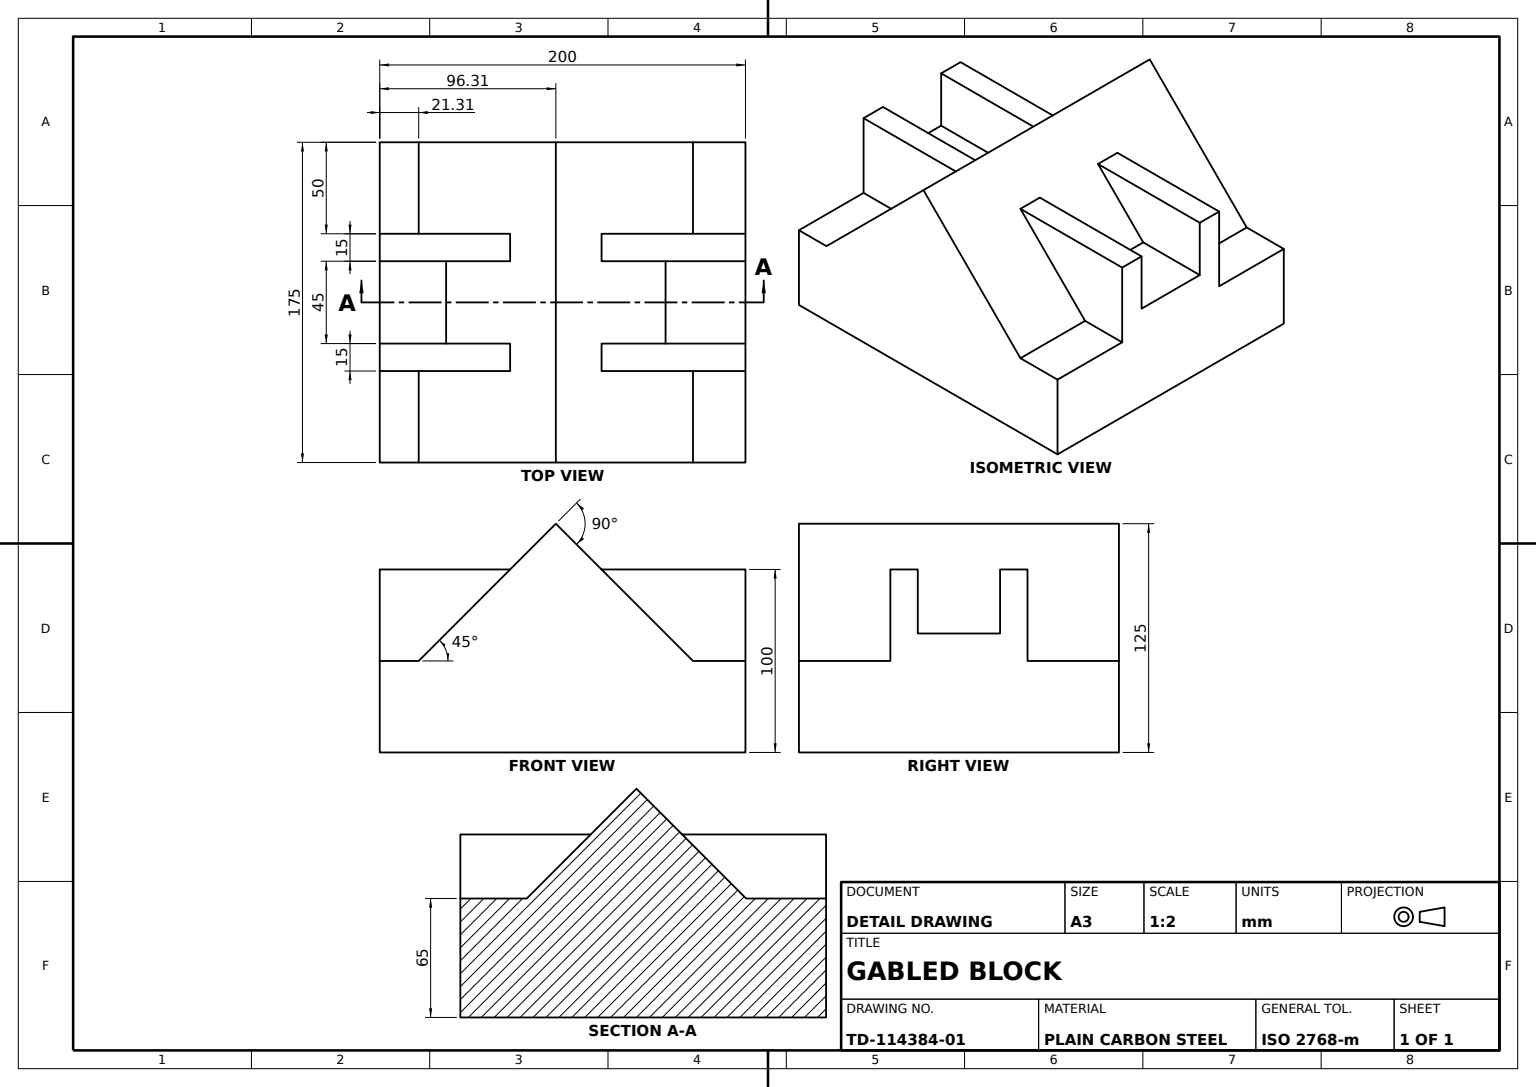
SolidWorks part; units mm, degrees
material "Plain Carbon Steel"
ref_plane "Front Plane" through (0, 0, 0) normal (0, 0, 1) x (1, 0, 0)
ref_plane "Top Plane" through (0, 0, 0) normal (0, 1, 0) x (1, 0, 0)
ref_plane "Right Plane" through (0, 0, 0) normal (1, 0, 0) x (0, 0, -1)
sketch "Base Profile Sketch" plane through (0, 0, 0) normal (0, 0, 1) x (1, 0, 0)
  line L1 (-103.689, 0) -> (103.689, 0) construction
  line L3 (-96.311, 0) -> (103.689, 0)
  line L4 (-96.311, 0) -> (-96.311, 50)
  line L5 (-96.311, 50) -> (-75, 50)
  line L6 (103.689, 0) -> (103.689, 50)
  line L7 (0, 125) -> (-75, 50)
  line L8 (0, 125) -> (75, 50)
  line L9 (75, 50) -> (103.689, 50)
  point P4 (0, 0)
  point P8 (0, 0)
  dimension "D1" = 200
  dimension "D2" = 50
  dimension "D3" = 21.311
  dimension "D4" = 90
  dimension "D5" = 96.311
extrude "Base Wedge Block" add sketch "Base Profile Sketch" along normal mid plane 175
sketch "Slot Profile Sketch" plane through (103.689, 0, 0) normal (1, 0, 0) x (0, 0, -1)
  line L0 (-87.5, 0) -> (-87.5, 50)
  line L1 (-87.5, 50) -> (-37.5, 50)
  line L2 (-87.5, 50) -> (87.5, 50) construction
  line L3 (-37.5, 50) -> (-37.5, 100)
  line L4 (-37.5, 100) -> (-22.5, 100)
  line L5 (-22.5, 100) -> (-22.5, 65)
  line L6 (-22.5, 65) -> (22.5, 65)
  line L7 (22.5, 65) -> (22.5, 100)
  line L8 (22.5, 100) -> (37.5, 100)
  line L9 (37.5, 100) -> (37.5, 50)
  line L10 (37.5, 50) -> (87.5, 50)
  line L11 (87.5, 50) -> (87.5, 0)
  line L12 (87.5, 0) -> (-87.5, 0)
  line L13 (0, 0) -> (0, 121.6217) construction
  dimension "D1" = 15
  dimension "D2" = 15
  dimension "D3" = 15
  dimension "D4" = 100
  dimension "D5" = 100
  dimension "D6" = 50
  dimension "D7" = 50
extrude "Twin Slots 15mm" add sketch "Slot Profile Sketch" against normal through all
